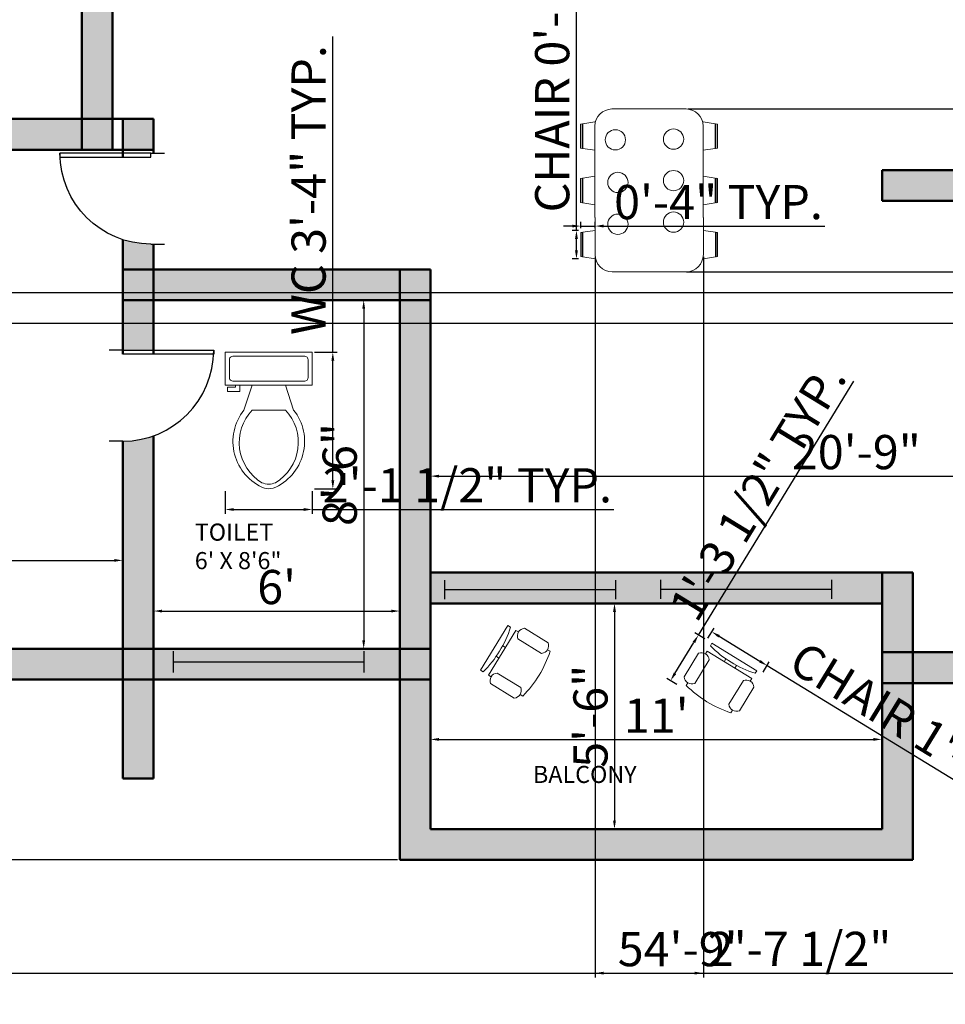
# Model space of a CAD drawing. Units: millimetres. Extents: x 2208 to 3043, y 878 to 1386.
# Tile 2 of 4: x 2479 to 2749, y 878 to 1166. Entities that reach past the tile are written whole.
import ezdxf

# ---------------------------------------------------------------- set-up
doc = ezdxf.new("R2010")
doc.units = ezdxf.units.MM
for name, color, linetype, lineweight in [('A-ANNO-DIMS', 50, 'Continuous', 13), ('A-AREA-IDEN', 90, 'Continuous', 25), ('A-FLOR-FIXT', 140, 'Continuous', 18), ('A-WALL-PATT', 6, 'Continuous', 13), ('doors', 30, 'Continuous', 25), ('furniture', 140, 'Continuous', 18), ('walls', 200, 'Continuous', 50), ('windows', 10, 'Continuous', 25)]:
    doc.layers.add(name, color=color, linetype=linetype, lineweight=lineweight)
doc.styles.get("Standard").update_dxf_attribs({"font": 'arial.ttf'})
doc.dimstyles.new('ISO-25', dxfattribs={"dimtxt": 10, "dimasz": 2.5, "dimexe": 1.25, "dimexo": 0.625, "dimtad": 1, "dimdec": 0, "dimlunit": 3, "dimtxsty": 'Standard', "dimcen": 2.5, "dimadec": 0, "dimazin": 0, "dimtfac": 1, "dimtdec": 0, "dimtmove": 0, "dimatfit": 3, "dimfxl": 1, "dimarcsym": 0})

# ---------------------------------------------------------------- blocks, each defined once
blk = doc.blocks.new('*U2')
for p, q in [((0, 0), (0, -6)), ((40, 0), (40, -6))]:
    blk.add_line(p, q)
blk.add_lwpolyline([(0, 0), (0, 40), (1.75, 40), (1.75, 0)], close=True)
blk.add_arc((0, 0), 40, 0, 90)
blk = doc.blocks.new('*U4')
for p, q in [((0, 4), (0, 0)), ((36, 4), (36, 0)), ((0, 2), (36, 2))]:
    blk.add_line(p, q)
blk = doc.blocks.new('*U5')
for p, q in [((0, 4), (0, 0)), ((36, 4), (36, 0)), ((0, 2), (36, 2))]:
    blk.add_line(p, q)
blk = doc.blocks.new('Chair - Desk')
for p, q in [((-8.5, 0), (-8.5, -1)), ((-8.5, 0), (8.5, 0)), ((8.5, 0), (8.5, -1)), ((-8.5, -3), (-8.5, -4)), ((-8.5, -3), (8.5, -3)), ((-2, -3), (-2, -1.9355)), ((2, -1.9576), (2, -3)), ((8.5, -3), (8.5, -4)), ((-10.5, -5), (-10.5, -14)), ((-6.5, -14), (-6.5, -5)), ((6.5, -5), (6.5, -14)), ((10.5, -14), (10.5, -5)), ((-8.5, -15), (-8.5, -16)), ((8.5, -15), (8.5, -16))]:
    blk.add_line(p, q)
for centre, radius, start, end in [((0, 34.625), 36.625, 256.5803, 283.4197), ((-8.5, -6.5), 2.5, 36.8699, 143.1301), ((8.5, -6.5), 2.5, 36.8699, 143.1301), ((-8.5, -12.5), 2.5, 216.8699, 323.1301), ((8.5, -12.5), 2.5, 216.8699, 323.1301), ((0, 19.625), 36.625, 256.5803, 283.4197)]:
    blk.add_arc(centre, radius, start, end)
blk = doc.blocks.new('Toilet - top')
for p, q in [((9.5, -6), (9.5, -2)), ((-10, -8.5), (-8, -8.5)), ((-10, -9.5), (-10, -8.5)), ((-7, -9.5), (-10, -9.5)), ((-8, -8.5), (-8, -8)), ((-7, -8), (-7, -9.5)), ((-4, -8), (-6, -14)), ((4, -8), (6, -14)), ((4, -14), (-4, -14))]:
    blk.add_line(p, q)
blk.add_lwpolyline([(10.5, -8), (10.5, 0), (-10.5, 0), (-10.5, -8)], close=True)
for points in [[(-9.5, -2), (-9.5, -6)], [(8.5, -1), (-8.5, -1)], [(-8.5, -7), (8.5, -7)]]:
    blk.add_lwpolyline(points)
for centre, radius, start, end in [((-8.62, -1.88), 0.884, 81.8699, 188.1301), ((8.62, -1.88), 0.884, 351.8699, 98.1301), ((-8.62, -6.12), 0.884, 171.8699, 278.1301), ((8.62, -6.12), 0.884, 261.8699, 8.1301), ((3.52, -21.58), 12.17, 141.4691, 247.9714), ((4.2, -21.82), 11.33, 136.3677, 238.9468), ((-3.52, -21.58), 12.17, 292.0284, 38.5307), ((-4.2, -21.82), 11.33, 301.053, 43.6321), ((0, -27.88), 4, 245.7318, 294.2682), ((0, -29), 4, 254.8605, 285.1395)]:
    blk.add_arc(centre, radius, start, end)
blk = doc.blocks.new('*D22')
at = {"layer": 'A-ANNO-DIMS', "color": 0, "lineweight": -2, "transparency": 16777216}
for p, q in [((2352.98, 996.86), (2352.98, 1009.56)), ((2355.48, 1008.31), (2506.48, 1008.31)), ((2508.98, 996.86), (2508.98, 1009.56))]:
    blk.add_line(p, q, dxfattribs=at)
at = {"layer": 'A-ANNO-DIMS', "color": 0, "transparency": 16777216}
for points in [[(2355.48, 1008.73), (2355.48, 1007.9), (2352.98, 1008.31)], [(2506.48, 1008.73), (2506.48, 1007.9), (2508.98, 1008.31)]]:
    blk.add_solid(points, dxfattribs=at)
at = {"layer": 'Defpoints', "color": 0, "transparency": 16777216}
for p in [(2508.98, 1008.31), (2352.98, 996.23), (2508.98, 996.23)]:
    blk.add_point(p, dxfattribs=at)
at = {"layer": 'A-ANNO-DIMS', "color": 0, "transparency": 16777216, "insert": (2430.98, 1014.05), "char_height": 10, "attachment_point": 5}
blk.add_mtext("13'", dxfattribs=at)
blk = doc.blocks.new('*D23')
at = {"layer": 'A-ANNO-DIMS', "color": 0, "lineweight": -2, "transparency": 16777216}
for p, q in [((2517.98, 1002.61), (2517.98, 992.24)), ((2589.98, 1002.61), (2589.98, 992.24)), ((2520.48, 993.49), (2587.48, 993.49))]:
    blk.add_line(p, q, dxfattribs=at)
at = {"layer": 'A-ANNO-DIMS', "color": 0, "transparency": 16777216}
for points in [[(2520.48, 993.9), (2520.48, 993.07), (2517.98, 993.49)], [(2587.48, 993.9), (2587.48, 993.07), (2589.98, 993.49)]]:
    blk.add_solid(points, dxfattribs=at)
at = {"layer": 'Defpoints', "color": 0, "transparency": 16777216}
for p in [(2517.98, 1003.23), (2589.98, 1003.23), (2589.98, 993.49)]:
    blk.add_point(p, dxfattribs=at)
at = {"layer": 'A-ANNO-DIMS', "color": 0, "transparency": 16777216, "insert": (2553.98, 999.22), "char_height": 10, "attachment_point": 5}
blk.add_mtext("6'", dxfattribs=at)
blk = doc.blocks.new('*D24')
at = {"layer": 'A-ANNO-DIMS', "color": 0, "lineweight": -2, "transparency": 16777216}
for p, q in [((2582.68, 1084.44), (2578.18, 1084.44)), ((2579.43, 1081.94), (2579.43, 984.94)), ((2582.68, 982.44), (2578.18, 982.44))]:
    blk.add_line(p, q, dxfattribs=at)
at = {"layer": 'A-ANNO-DIMS', "color": 0, "transparency": 16777216}
for points in [[(2579.01, 1081.94), (2579.85, 1081.94), (2579.43, 1084.44)], [(2579.01, 984.94), (2579.85, 984.94), (2579.43, 982.44)]]:
    blk.add_solid(points, dxfattribs=at)
at = {"layer": 'Defpoints', "color": 0, "transparency": 16777216}
for p in [(2583.3, 1084.44), (2579.43, 982.44), (2583.3, 982.44)]:
    blk.add_point(p, dxfattribs=at)
at = {"layer": 'A-ANNO-DIMS', "color": 0, "transparency": 16777216, "insert": (2573.7, 1033.44), "char_height": 10, "attachment_point": 5, "rotation": 90}
blk.add_mtext('8\'-6"', dxfattribs=at)
blk = doc.blocks.new('*D25')
at = {"layer": 'A-ANNO-DIMS', "color": 0, "lineweight": -2, "transparency": 16777216}
for p, q in [((2598.98, 952.2), (2598.98, 957.19)), ((2730.98, 952.2), (2730.98, 957.19)), ((2601.48, 955.94), (2728.48, 955.94))]:
    blk.add_line(p, q, dxfattribs=at)
at = {"layer": 'A-ANNO-DIMS', "color": 0, "transparency": 16777216}
for points in [[(2601.48, 956.36), (2601.48, 955.53), (2598.98, 955.94)], [(2728.48, 956.36), (2728.48, 955.53), (2730.98, 955.94)]]:
    blk.add_solid(points, dxfattribs=at)
at = {"layer": 'Defpoints', "color": 0, "transparency": 16777216}
for p in [(2730.98, 955.94), (2598.98, 951.58), (2730.98, 951.58)]:
    blk.add_point(p, dxfattribs=at)
at = {"layer": 'A-ANNO-DIMS', "color": 0, "transparency": 16777216, "insert": (2664.98, 961.59), "char_height": 10, "attachment_point": 5}
blk.add_mtext("11'", dxfattribs=at)
blk = doc.blocks.new('*D26')
at = {"layer": 'A-ANNO-DIMS', "color": 0, "lineweight": -2, "transparency": 16777216}
for p, q in [((2657.86, 995.72), (2651.51, 995.72)), ((2652.76, 993.22), (2652.76, 932.22)), ((2657.86, 929.72), (2651.51, 929.72))]:
    blk.add_line(p, q, dxfattribs=at)
at = {"layer": 'A-ANNO-DIMS', "color": 0, "transparency": 16777216}
for points in [[(2652.34, 993.22), (2653.18, 993.22), (2652.76, 995.72)], [(2652.34, 932.22), (2653.18, 932.22), (2652.76, 929.72)]]:
    blk.add_solid(points, dxfattribs=at)
at = {"layer": 'Defpoints', "color": 0, "transparency": 16777216}
for p in [(2658.49, 995.72), (2652.76, 929.72), (2658.49, 929.72)]:
    blk.add_point(p, dxfattribs=at)
at = {"layer": 'A-ANNO-DIMS', "color": 0, "transparency": 16777216, "insert": (2647.03, 962.72), "char_height": 10, "attachment_point": 5, "rotation": 90}
blk.add_mtext('5\'-6"', dxfattribs=at)
blk = doc.blocks.new('*D27')
at = {"layer": 'A-ANNO-DIMS', "color": 0, "lineweight": -2, "transparency": 16777216}
for p, q in [((2598.98, 1051.4), (2598.98, 1031.71)), ((2847.98, 1051.4), (2847.98, 1031.71)), ((2601.48, 1032.96), (2845.48, 1032.96))]:
    blk.add_line(p, q, dxfattribs=at)
at = {"layer": 'A-ANNO-DIMS', "color": 0, "transparency": 16777216}
for points in [[(2601.48, 1033.38), (2601.48, 1032.54), (2598.98, 1032.96)], [(2845.48, 1033.38), (2845.48, 1032.54), (2847.98, 1032.96)]]:
    blk.add_solid(points, dxfattribs=at)
at = {"layer": 'Defpoints', "color": 0, "transparency": 16777216}
for p in [(2598.98, 1052.02), (2847.98, 1052.02), (2847.98, 1032.96)]:
    blk.add_point(p, dxfattribs=at)
at = {"layer": 'A-ANNO-DIMS', "color": 0, "transparency": 16777216, "insert": (2723.48, 1038.69), "char_height": 10, "attachment_point": 5}
blk.add_mtext('20\'-9"', dxfattribs=at)
blk = doc.blocks.new('CHAIR-DINING')
for p, q in [((0, 7.69), (0.44, 7.76)), ((0, 7.69), (0, 0.65)), ((0.44, 0.58), (0.44, 7.76)), ((0.66, 7.79), (4.18, 8.34)), ((0.66, 7.79), (0.66, 0.55)), ((0.44, 0.58), (0, 0.65)), ((4.18, 0), (0.66, 0.55))]:
    blk.add_line(p, q)
blk = doc.blocks.new('*D34')
at = {"layer": 'A-ANNO-DIMS', "color": 0, "lineweight": -2, "transparency": 16777216}
for p, q in [((2641.64, 1104.85), (2641.64, 1240.09)), ((2642.27, 1104.85), (2640.39, 1104.85)), ((2641.64, 1099.01), (2641.64, 1102.35)), ((2642.27, 1096.51), (2640.39, 1096.51))]:
    blk.add_line(p, q, dxfattribs=at)
at = {"layer": 'A-ANNO-DIMS', "color": 0, "transparency": 16777216}
for points in [[(2641.22, 1102.35), (2642.06, 1102.35), (2641.64, 1104.85)], [(2641.22, 1099.01), (2642.06, 1099.01), (2641.64, 1096.51)]]:
    blk.add_solid(points, dxfattribs=at)
at = {"layer": 'Defpoints', "color": 0, "transparency": 16777216}
for p in [(2641.64, 1104.85), (2642.89, 1104.85), (2642.89, 1096.51)]:
    blk.add_point(p, dxfattribs=at)
at = {"layer": 'A-ANNO-DIMS', "color": 0, "transparency": 16777216, "insert": (2635.84, 1173.72), "char_height": 10, "attachment_point": 5, "rotation": 90}
blk.add_mtext('CHAIR 0\'-8 1/2" TYP.', dxfattribs=at)
blk = doc.blocks.new('*D35')
at = {"layer": 'A-ANNO-DIMS', "color": 0, "lineweight": -2, "transparency": 16777216}
for p, q in [((2640.39, 1106.1), (2637.89, 1106.1)), ((2642.89, 1105.48), (2642.89, 1107.35)), ((2642.89, 1106.1), (2647.07, 1106.1)), ((2647.07, 1105.48), (2647.07, 1107.35)), ((2649.57, 1106.1), (2714.28, 1106.1))]:
    blk.add_line(p, q, dxfattribs=at)
at = {"layer": 'A-ANNO-DIMS', "color": 0, "transparency": 16777216}
for points in [[(2640.39, 1106.52), (2640.39, 1105.69), (2642.89, 1106.1)], [(2649.57, 1106.52), (2649.57, 1105.69), (2647.07, 1106.1)]]:
    blk.add_solid(points, dxfattribs=at)
at = {"layer": 'Defpoints', "color": 0, "transparency": 16777216}
for p in [(2647.07, 1106.1), (2642.89, 1104.85), (2647.07, 1104.85)]:
    blk.add_point(p, dxfattribs=at)
at = {"layer": 'A-ANNO-DIMS', "color": 0, "transparency": 16777216, "insert": (2683.17, 1111.83), "char_height": 10, "attachment_point": 5}
blk.add_mtext('0\'-4" TYP.', dxfattribs=at)
blk = doc.blocks.new('*D38')
at = {"layer": 'A-ANNO-DIMS', "color": 0, "lineweight": -2, "transparency": 16777216}
for p, q in [((2680.05, 985.52), (2681.86, 988.48)), ((2683.34, 986.11), (2695.25, 978.83)), ((2696.22, 975.63), (2698.03, 978.59)), ((2697.38, 977.52), (2792.87, 919.11))]:
    blk.add_line(p, q, dxfattribs=at)
at = {"layer": 'A-ANNO-DIMS', "color": 0, "transparency": 16777216}
for points in [[(2683.56, 986.47), (2683.13, 985.76), (2681.21, 987.42)], [(2695.47, 979.18), (2695.03, 978.47), (2697.38, 977.52)]]:
    blk.add_solid(points, dxfattribs=at)
at = {"layer": 'Defpoints', "color": 0, "transparency": 16777216}
for p in [(2679.73, 984.99), (2697.38, 977.52), (2695.9, 975.1)]:
    blk.add_point(p, dxfattribs=at)
at = {"layer": 'A-ANNO-DIMS', "color": 0, "transparency": 16777216, "insert": (2749.21, 952.61), "char_height": 10, "attachment_point": 5, "rotation": 328.5439}
blk.add_mtext('CHAIR 1\'-7" TYP.', dxfattribs=at)
blk = doc.blocks.new('*D39')
at = {"layer": 'A-ANNO-DIMS', "color": 0, "lineweight": -2, "transparency": 16777216}
for p, q in [((2677.3, 986.48), (2722.74, 1060.75)), ((2679.19, 985.32), (2676.24, 987.13)), ((2670.44, 975.26), (2676, 984.34)), ((2671.03, 971.97), (2668.07, 973.78))]:
    blk.add_line(p, q, dxfattribs=at)
at = {"layer": 'A-ANNO-DIMS', "color": 0, "transparency": 16777216}
for points in [[(2675.64, 984.56), (2676.35, 984.13), (2677.3, 986.48)], [(2670.09, 975.48), (2670.8, 975.04), (2669.14, 973.13)]]:
    blk.add_solid(points, dxfattribs=at)
at = {"layer": 'Defpoints', "color": 0, "transparency": 16777216}
for p in [(2677.3, 986.48), (2679.73, 984.99), (2671.56, 971.64)]:
    blk.add_point(p, dxfattribs=at)
at = {"layer": 'A-ANNO-DIMS', "color": 0, "transparency": 16777216, "insert": (2695.72, 1027.7), "char_height": 10, "attachment_point": 5, "rotation": 58.5439}
blk.add_mtext('1\'-3 1/2" TYP.', dxfattribs=at)
blk = doc.blocks.new('*D40')
at = {"layer": 'A-ANNO-DIMS', "color": 0, "lineweight": -2, "transparency": 16777216}
for p, q in [((2570.4, 1069.24), (2570.4, 1161.51)), ((2565.02, 1069.24), (2571.65, 1069.24)), ((2570.4, 1031.7), (2570.4, 1066.74)), ((2565.02, 1029.2), (2571.65, 1029.2))]:
    blk.add_line(p, q, dxfattribs=at)
at = {"layer": 'A-ANNO-DIMS', "color": 0, "transparency": 16777216}
for points in [[(2569.99, 1066.74), (2570.82, 1066.74), (2570.4, 1069.24)], [(2569.99, 1031.7), (2570.82, 1031.7), (2570.4, 1029.2)]]:
    blk.add_solid(points, dxfattribs=at)
at = {"layer": 'Defpoints', "color": 0, "transparency": 16777216}
for p in [(2564.4, 1069.24), (2570.4, 1069.24), (2564.4, 1029.2)]:
    blk.add_point(p, dxfattribs=at)
at = {"layer": 'A-ANNO-DIMS', "color": 0, "transparency": 16777216, "insert": (2564.61, 1116.63), "char_height": 10, "attachment_point": 5, "rotation": 90}
blk.add_mtext('WC 3\'-4" TYP.', dxfattribs=at)
blk = doc.blocks.new('*D41')
at = {"layer": 'A-ANNO-DIMS', "color": 0, "lineweight": -2, "transparency": 16777216}
for p, q in [((2538.95, 1028.57), (2538.95, 1021.94)), ((2564.4, 1028.57), (2564.4, 1021.94)), ((2541.45, 1023.19), (2561.9, 1023.19)), ((2564.4, 1023.19), (2652.58, 1023.19))]:
    blk.add_line(p, q, dxfattribs=at)
at = {"layer": 'A-ANNO-DIMS', "color": 0, "transparency": 16777216}
for points in [[(2541.45, 1023.61), (2541.45, 1022.78), (2538.95, 1023.19)], [(2561.9, 1023.61), (2561.9, 1022.78), (2564.4, 1023.19)]]:
    blk.add_solid(points, dxfattribs=at)
at = {"layer": 'Defpoints', "color": 0, "transparency": 16777216}
for p in [(2538.95, 1029.2), (2564.4, 1029.2), (2564.4, 1023.19)]:
    blk.add_point(p, dxfattribs=at)
at = {"layer": 'A-ANNO-DIMS', "color": 0, "transparency": 16777216, "insert": (2609.74, 1028.99), "char_height": 10, "attachment_point": 5}
blk.add_mtext('2\'-1 1/2" TYP.', dxfattribs=at)
blk = doc.blocks.new('*D46')
at = {"layer": 'A-ANNO-DIMS', "color": 0, "lineweight": -2, "transparency": 16777216}
for p, q in [((3001.16, 1077), (3001.16, 886.32)), ((2343.98, 972.81), (2343.98, 886.32)), ((2346.48, 887.57), (2998.66, 887.57))]:
    blk.add_line(p, q, dxfattribs=at)
at = {"layer": 'A-ANNO-DIMS', "color": 0, "transparency": 16777216}
for points in [[(2346.48, 887.99), (2346.48, 887.16), (2343.98, 887.57)], [(2998.66, 887.99), (2998.66, 887.16), (3001.16, 887.57)]]:
    blk.add_solid(points, dxfattribs=at)
at = {"layer": 'Defpoints', "color": 0, "transparency": 16777216}
for p in [(3001.16, 1077.62), (2343.98, 973.44), (3001.16, 887.57)]:
    blk.add_point(p, dxfattribs=at)
at = {"layer": 'A-ANNO-DIMS', "color": 0, "transparency": 16777216, "insert": (2672.57, 893.3), "char_height": 10, "attachment_point": 5}
blk.add_mtext('54\'-9"', dxfattribs=at)
blk = doc.blocks.new('*D47')
at = {"layer": 'A-ANNO-DIMS', "color": 0, "lineweight": -2, "transparency": 16777216}
for p, q in [((2343.36, 1332.44), (2309.12, 1332.44)), ((2310.37, 1329.94), (2310.37, 923.22)), ((2589.36, 920.72), (2309.12, 920.72))]:
    blk.add_line(p, q, dxfattribs=at)
at = {"layer": 'A-ANNO-DIMS', "color": 0, "transparency": 16777216}
for points in [[(2309.95, 1329.94), (2310.79, 1329.94), (2310.37, 1332.44)], [(2309.95, 923.22), (2310.79, 923.22), (2310.37, 920.72)]]:
    blk.add_solid(points, dxfattribs=at)
at = {"layer": 'Defpoints', "color": 0, "transparency": 16777216}
for p in [(2343.98, 1332.44), (2310.37, 920.72), (2589.98, 920.72)]:
    blk.add_point(p, dxfattribs=at)
at = {"layer": 'A-ANNO-DIMS', "color": 0, "transparency": 16777216, "insert": (2304.57, 1126.58), "char_height": 10, "attachment_point": 5, "rotation": 90}
blk.add_mtext('34\'-3 1/2"', dxfattribs=at)
blk = doc.blocks.new('*D62')
at = {"layer": 'A-ANNO-DIMS', "color": 0, "lineweight": -2, "transparency": 16777216}
for p, q in [((2310.37, 1086.62), (2310.37, 1116.95)), ((3000.54, 1086.62), (2309.12, 1086.62)), ((2310.37, 1080.12), (2310.37, 1084.12)), ((3000.54, 1077.62), (2309.12, 1077.62))]:
    blk.add_line(p, q, dxfattribs=at)
at = {"layer": 'A-ANNO-DIMS', "color": 0, "transparency": 16777216}
for points in [[(2309.95, 1084.12), (2310.79, 1084.12), (2310.37, 1086.62)], [(2309.95, 1080.12), (2310.79, 1080.12), (2310.37, 1077.62)]]:
    blk.add_solid(points, dxfattribs=at)
at = {"layer": 'Defpoints', "color": 0, "transparency": 16777216}
for p in [(2310.37, 1086.62), (3001.16, 1086.62), (3001.16, 1077.62)]:
    blk.add_point(p, dxfattribs=at)
at = {"layer": 'A-ANNO-DIMS', "color": 0, "transparency": 16777216, "insert": (2304.64, 1103.04), "char_height": 10, "attachment_point": 5, "rotation": 90}
blk.add_mtext('0\'-9"', dxfattribs=at)
blk = doc.blocks.new('*D65')
at = {"layer": 'A-ANNO-DIMS', "color": 0, "lineweight": -2, "transparency": 16777216}
for p, q in [((2647.07, 1097.14), (2647.07, 886.32)), ((2678.74, 1097.14), (2678.74, 886.32)), ((2649.57, 887.57), (2676.24, 887.57)), ((2678.74, 887.57), (2732.54, 887.57))]:
    blk.add_line(p, q, dxfattribs=at)
at = {"layer": 'A-ANNO-DIMS', "color": 0, "transparency": 16777216}
for points in [[(2649.57, 887.99), (2649.57, 887.16), (2647.07, 887.57)], [(2676.24, 887.99), (2676.24, 887.16), (2678.74, 887.57)]]:
    blk.add_solid(points, dxfattribs=at)
at = {"layer": 'Defpoints', "color": 0, "transparency": 16777216}
for p in [(2647.07, 1097.76), (2678.74, 1097.76), (2678.74, 887.57)]:
    blk.add_point(p, dxfattribs=at)
at = {"layer": 'A-ANNO-DIMS', "color": 0, "transparency": 16777216, "insert": (2706.89, 893.37), "char_height": 10, "attachment_point": 5}
blk.add_mtext('2\'-7 1/2"', dxfattribs=at)
blk = doc.blocks.new('*D66')
at = {"layer": 'A-ANNO-DIMS', "color": 0, "lineweight": -2, "transparency": 16777216}
for p, q in [((3034.31, 1140.35), (3034.31, 1201.74)), ((2674.33, 1140.35), (3035.56, 1140.35)), ((3034.31, 1095.26), (3034.31, 1137.85)), ((2673.86, 1092.76), (3035.56, 1092.76))]:
    blk.add_line(p, q, dxfattribs=at)
at = {"layer": 'A-ANNO-DIMS', "color": 0, "transparency": 16777216}
for points in [[(3033.9, 1137.85), (3034.73, 1137.85), (3034.31, 1140.35)], [(3033.9, 1095.26), (3034.73, 1095.26), (3034.31, 1092.76)]]:
    blk.add_solid(points, dxfattribs=at)
at = {"layer": 'Defpoints', "color": 0, "transparency": 16777216}
for p in [(2673.7, 1140.35), (3034.31, 1140.35), (2673.23, 1092.76)]:
    blk.add_point(p, dxfattribs=at)
at = {"layer": 'A-ANNO-DIMS', "color": 0, "transparency": 16777216, "insert": (3028.52, 1172.3), "char_height": 10, "attachment_point": 5, "rotation": 90}
blk.add_mtext('3\'-11 1/2"', dxfattribs=at)

msp = doc.modelspace()

# ---------------------------------------------------------------- hatches: boundary and pattern name
at = {"layer": 'A-WALL-PATT'}
h = msp.add_hatch(color=256, dxfattribs=at)
h.dxf.hatch_style = 1
h.paths.add_polyline_path([(2352.98, 1273, -0.051847), (2347.51, 1272.43), (2343.98, 1272.43), (2343.98, 1137.44), (2352.98, 1137.44)])
h.paths.add_polyline_path([(2352.98, 1323.44), (2343.98, 1323.44), (2343.98, 1299.03), (2347.51, 1299.03), (2352.98, 1299.03)])
h.paths.add_polyline_path([(2352.98, 1332.44), (2343.98, 1332.44), (2343.98, 1323.44), (2352.98, 1323.44)])
h.paths.add_polyline_path([(2496.98, 1332.44), (2352.98, 1332.44), (2352.98, 1323.44), (2496.98, 1323.44)])
h.paths.add_polyline_path([(2505.98, 1323.44), (2496.98, 1323.44), (2496.98, 1191.44), (2505.98, 1191.44)])
h.paths.add_polyline_path([(2505.98, 1332.44), (2496.98, 1332.44), (2496.98, 1323.44), (2505.98, 1323.44)])
h.paths.add_polyline_path([(2505.98, 1182.44), (2496.98, 1182.44), (2496.98, 1137.44), (2505.98, 1137.44)])
h.paths.add_polyline_path([(2505.98, 1191.44), (2496.98, 1191.44), (2496.98, 1182.44), (2505.98, 1182.44)])
h.paths.add_polyline_path([(2621.06, 1191.44), (2505.98, 1191.44), (2505.98, 1182.44), (2619.92, 1182.44), (2619.92, 1183.73, -0.073589)])
h.paths.add_polyline_path([(2496.98, 1137.44), (2352.98, 1137.44), (2352.98, 1128.44), (2496.98, 1128.44)])
h.paths.add_polyline_path([(2352.98, 1137.44), (2343.98, 1137.44), (2343.98, 1128.44), (2352.98, 1128.44)])
h.paths.add_polyline_path([(2352.98, 1128.44), (2343.98, 1128.44), (2343.98, 982.44), (2352.98, 982.44)])
h.paths.add_polyline_path([(2517.98, 1137.44), (2508.98, 1137.44), (2508.98, 1128.44), (2517.98, 1128.44)])
h.paths.add_polyline_path([(2505.98, 1137.44), (2496.98, 1137.44), (2496.98, 1128.44), (2505.98, 1128.44)])
h.paths.add_polyline_path([(2658.98, 1224.44), (2649.98, 1224.44), (2649.98, 1191.44), (2658.98, 1191.44)])
h.paths.add_polyline_path([(2658.98, 1323.44), (2649.98, 1323.44), (2649.98, 1233.44), (2658.98, 1233.44)])
h.paths.add_polyline_path([(2658.98, 1233.44), (2649.98, 1233.44), (2649.98, 1224.44), (2658.98, 1224.44)])
h.paths.add_polyline_path([(2730.98, 1233.44), (2658.98, 1233.44), (2658.98, 1224.44), (2730.98, 1224.44)])
h.paths.add_polyline_path([(2739.98, 1323.44), (2730.98, 1323.44), (2730.98, 1233.44), (2739.98, 1233.44)])
h.paths.add_polyline_path([(2739.98, 1224.44), (2730.98, 1224.44), (2730.98, 1191.44), (2739.98, 1191.44)])
h.paths.add_polyline_path([(2739.98, 1191.44), (2730.98, 1191.44), (2730.98, 1182.44), (2739.98, 1182.44)])
h.paths.add_polyline_path([(2739.98, 1182.44), (2730.98, 1182.44), (2730.98, 1171.44), (2739.98, 1171.44)])
h.paths.add_polyline_path([(2739.98, 972.44), (2730.98, 972.44), (2730.98, 929.72), (2602.15, 929.72), (2598.98, 929.72), (2598.98, 973.44), (2589.98, 973.44), (2589.98, 929.72), (2589.98, 920.72), (2730.98, 920.72), (2739.98, 920.72)])
h.paths.add_polyline_path([(2598.98, 1084.44), (2589.98, 1084.44), (2589.98, 982.44), (2598.98, 982.44)])
h.paths.add_polyline_path([(2598.98, 982.44), (2589.98, 982.44), (2589.98, 973.44), (2598.98, 973.44)])
h.paths.add_polyline_path([(2517.98, 973.44), (2508.98, 973.44), (2508.98, 944.53), (2517.98, 944.53)])
h.paths.add_polyline_path([(2517.98, 1044.76, -0.086498), (2508.98, 1043.19), (2508.98, 982.44), (2517.98, 982.44)])
h.paths.add_polyline_path([(2517.98, 982.44), (2508.98, 982.44), (2508.98, 973.44), (2517.98, 973.44)])
h.paths.add_polyline_path([(2352.98, 982.44), (2343.98, 982.44), (2343.98, 973.44), (2352.98, 973.44)])
h.paths.add_polyline_path([(2589.98, 1093.44), (2517.98, 1093.44), (2517.98, 1084.44), (2589.98, 1084.44)])
h.paths.add_polyline_path([(2517.98, 1093.44), (2508.98, 1093.44), (2508.98, 1084.44), (2517.98, 1084.44)])
h.paths.add_polyline_path([(2517.98, 1084.44), (2508.98, 1084.44), (2508.98, 1069.79), (2517.98, 1069.79)])
h.paths.add_polyline_path([(2517.98, 1100.83), (2517.21, 1100.83, -0.078775), (2508.98, 1102.14), (2508.98, 1093.44), (2517.98, 1093.44)])
h.paths.add_polyline_path([(2598.98, 1093.44), (2589.98, 1093.44), (2589.98, 1084.44), (2598.98, 1084.44)])
h.paths.add_polyline_path([(2802.98, 1122.44), (2730.98, 1122.44), (2730.98, 1113.44), (2802.98, 1113.44)])
h.paths.add_polyline_path([(2922.98, 1113.44), (2913.98, 1113.44), (2913.98, 981.44), (2922.98, 981.44)])
h.paths.add_polyline_path([(2856.98, 1069.77, -0.087206), (2847.98, 1067.81), (2847.98, 981.44), (2856.98, 981.44)])
h.paths.add_polyline_path([(2913.98, 981.44), (2856.98, 981.44), (2856.98, 972.44), (2913.98, 972.44)])
h.paths.add_polyline_path([(2856.98, 981.44), (2847.98, 981.44), (2847.98, 972.44), (2856.98, 972.44)])
h.paths.add_polyline_path([(2739.98, 995.72), (2739.98, 1004.72), (2730.98, 1004.72), (2730.98, 981.44), (2739.98, 981.44)])
h.paths.add_polyline_path([(2739.98, 981.44), (2730.98, 981.44), (2730.98, 972.44), (2739.98, 972.44)])
h.paths.add_polyline_path([(2922.98, 981.44), (2913.98, 981.44), (2913.98, 972.44), (2922.98, 972.44)])
h.paths.add_polyline_path([(3001.16, 1086.62), (2922.98, 1086.62), (2922.98, 1077.62), (3001.16, 1077.62)])
h.paths.add_polyline_path([(3001.16, 1191.44), (2922.98, 1191.44), (2922.98, 1182.44), (3001.16, 1182.44)])
h.paths.add_polyline_path([(2913.98, 1191.44), (2843.61, 1191.44), (2843.49, 1188.69, -0.05974), (2842.46, 1182.44), (2913.98, 1182.44)])
h.paths.add_polyline_path([(2922.98, 1191.44), (2913.98, 1191.44), (2913.98, 1182.44), (2922.98, 1182.44)])
h.paths.add_polyline_path([(2802.98, 1191.44), (2769.17, 1191.44, -0.079558), (2770.5, 1183.13), (2770.5, 1182.44), (2802.98, 1182.44)])
h.paths.add_polyline_path([(2811.98, 1191.44), (2802.98, 1191.44), (2802.98, 1182.44), (2811.98, 1182.44)])
h.paths.add_polyline_path([(2811.98, 1182.44), (2802.98, 1182.44), (2802.98, 1122.44), (2811.98, 1122.44)])
h.paths.add_polyline_path([(2811.98, 1122.44), (2802.98, 1122.44), (2802.98, 1113.44), (2811.98, 1113.44)])
h.paths.add_polyline_path([(2847.98, 1122.44), (2811.98, 1122.44), (2811.98, 1113.44), (2847.98, 1113.44)])
h.paths.add_polyline_path([(2856.98, 1122.44), (2847.98, 1122.44), (2847.98, 1113.44), (2856.98, 1113.44)])
h.paths.add_polyline_path([(2913.98, 1122.44), (2856.98, 1122.44), (2856.98, 1113.44), (2913.98, 1113.44)])
h.paths.add_polyline_path([(2922.98, 1122.44), (2913.98, 1122.44), (2913.98, 1113.44), (2922.98, 1113.44)])
h.paths.add_polyline_path([(2856.98, 1113.44), (2847.98, 1113.44), (2847.98, 1094.39), (2856.98, 1094.39)])
h.paths.add_polyline_path([(2922.98, 1323.44), (2913.98, 1323.44), (2913.98, 1191.44), (2922.98, 1191.44)])
h.paths.add_polyline_path([(2922.98, 1332.44), (2913.98, 1332.44), (2913.98, 1323.44), (2922.98, 1323.44)])
h.paths.add_polyline_path([(2913.98, 1332.44), (2739.98, 1332.44), (2739.98, 1323.44), (2913.98, 1323.44)])
h.paths.add_polyline_path([(2730.98, 1332.44), (2658.98, 1332.44), (2658.98, 1323.44), (2730.98, 1323.44)])
h.paths.add_polyline_path([(2649.98, 1332.44), (2505.98, 1332.44), (2505.98, 1323.44), (2649.98, 1323.44)])
h.paths.add_polyline_path([(2658.98, 1332.44), (2649.98, 1332.44), (2649.98, 1323.44), (2658.98, 1323.44)])
h.paths.add_polyline_path([(2739.98, 1332.44), (2730.98, 1332.44), (2730.98, 1323.44), (2739.98, 1323.44)])
h.paths.add_polyline_path([(2739.98, 1233.44), (2730.98, 1233.44), (2730.98, 1224.44), (2739.98, 1224.44)])
h.paths.add_polyline_path([(2658.98, 1191.44), (2649.98, 1191.44), (2649.98, 1182.44), (2658.98, 1182.44)])
h.paths.add_polyline_path([(2658.98, 1182.44), (2649.98, 1182.44), (2649.98, 1171.44), (2658.98, 1171.44)])
h.paths.add_polyline_path([(2508.98, 982.44), (2352.98, 982.44), (2352.98, 973.44), (2508.98, 973.44)])
h.paths.add_polyline_path([(2589.98, 982.44), (2517.98, 982.44), (2517.98, 973.44), (2589.98, 973.44)])
h.paths.add_polyline_path([(2730.98, 1004.72), (2598.98, 1004.72), (2598.98, 995.72), (2730.98, 995.72)])
h.paths.add_polyline_path([(2847.98, 981.44), (2739.98, 981.44), (2739.98, 972.44), (2847.98, 972.44)])

# ---------------------------------------------------------------- linework, layer by layer
at = {"layer": 'furniture'}
for p, q in [((2673.7, 1140.35), (2652.03, 1140.35)), ((2647.03, 1135.35), (2647.03, 1124.51)), ((2678.7, 1124.51), (2678.7, 1135.35)), ((2647.05, 1124.44), (2647.05, 1108.61)), ((2678.71, 1108.61), (2678.71, 1124.44)), ((2647.07, 1108.6), (2647.07, 1097.76)), ((2678.74, 1097.76), (2678.74, 1108.6)), ((2652.07, 1092.76), (2673.74, 1092.76)), ((2652.57, 1092.76), (2652.57, 1092.76)), ((2660.92, 1092.76), (2660.92, 1092.76)), ((2664.89, 1092.76), (2664.89, 1092.76)), ((2673.23, 1092.76), (2673.23, 1092.76))]:
    msp.add_line(p, q, dxfattribs=at)
for centre in [(2653.02, 1131.33), (2670.03, 1131.54), (2653.76, 1118.87), (2670.03, 1119.4), (2653.76, 1106.63), (2670.03, 1107.26)]:
    msp.add_circle(centre, 2.97, dxfattribs=at)
for centre, start, end in [((2652.03, 1135.35), 90, 180), ((2673.7, 1135.35), 0, 90), ((2652.07, 1097.76), 180, 270), ((2673.74, 1097.76), 270, 0)]:
    msp.add_arc(centre, 5, start, end, dxfattribs=at)
at = {"layer": 'walls'}
for p, q in [((2496.98, 1332.44), (2496.98, 1128.44)), ((2505.98, 1332.44), (2505.98, 1128.44)), ((2343.98, 1137.44), (2517.98, 1137.44)), ((2508.98, 1137.44), (2508.98, 1126.27)), ((2517.98, 1137.44), (2517.98, 1127.43)), ((2343.98, 1128.44), (2517.98, 1128.44)), ((2730.98, 1122.44), (2922.98, 1122.44)), ((2730.98, 1122.44), (2730.98, 1113.44)), ((2730.98, 1113.44), (2922.98, 1113.44)), ((2508.98, 1102.14), (2508.98, 1068.63)), ((2517.98, 1100.83), (2517.98, 1068.63)), ((2508.98, 1093.44), (2598.98, 1093.44)), ((2589.98, 1093.44), (2589.98, 973.44)), ((2598.98, 1093.44), (2598.98, 973.44)), ((2508.98, 1084.44), (2598.98, 1084.44)), ((2508.98, 1043.19), (2508.98, 973.44)), ((2517.98, 1044.76), (2517.98, 973.44)), ((2739.98, 1004.72), (2598.98, 1004.72)), ((2730.98, 1004.72), (2730.98, 972.44)), ((2739.98, 995.72), (2739.98, 1004.72)), ((2730.98, 995.72), (2598.98, 995.72)), ((2730.98, 995.72), (2730.98, 929.72)), ((2739.98, 995.72), (2739.98, 920.72)), ((2343.98, 982.44), (2598.98, 982.44)), ((2730.98, 981.44), (2922.98, 981.44)), ((2739.98, 981.44), (2739.98, 972.44)), ((2343.98, 973.44), (2598.98, 973.44)), ((2508.98, 973.44), (2508.98, 944.53)), ((2517.98, 973.44), (2517.98, 944.53)), ((2589.98, 929.72), (2589.98, 973.44)), ((2598.98, 929.72), (2598.98, 973.44)), ((2730.98, 972.44), (2922.98, 972.44)), ((2508.98, 944.53), (2517.98, 944.53)), ((2589.98, 929.72), (2589.98, 920.72)), ((2602.15, 929.72), (2598.98, 929.72)), ((2730.98, 929.72), (2602.15, 929.72)), ((2730.98, 920.72), (2589.98, 920.72)), ((2730.98, 920.72), (2739.98, 920.72))]:
    msp.add_line(p, q, dxfattribs=at)

# ---------------------------------------------------------------- block references
at = {"layer": 'A-FLOR-FIXT', "xscale": 1.211687514206988, "yscale": 1.211687514206988, "zscale": 1.211687514206988}
msp.add_blockref('Toilet - top', (2551.68, 1069.24), dxfattribs=at)
at = {"layer": 'doors', "yscale": 0.6650461219051067, "zscale": 0.6650461219051067}
for p, xscale, rotation in [((2517.21, 1127.43), -0.6650461219051067, 90), ((2508.98, 1069.79), 0.6650461219051067, 270)]:
    msp.add_blockref('*U2', p, dxfattribs=dict(at, xscale=xscale, rotation=rotation))
at = {"layer": 'furniture'}
for p in [(2642.85, 1128.26), (2642.87, 1112.35), (2642.89, 1096.51)]:
    msp.add_blockref('CHAIR-DINING', p, dxfattribs=at)
at = {"layer": 'furniture', "extrusion": (0, 0, -1), "zscale": -1, "rotation": 359.9999732726573}
for p in [(-2682.88, 1128.26), (-2682.89, 1112.35), (-2682.92, 1096.51)]:
    msp.add_blockref('CHAIR-DINING', p, dxfattribs=at)
at = {"layer": 'furniture'}
for p, xscale, yscale, zscale, rotation in [((2617.62, 982.71), 0.9026745047030139, 0.9026745047030139, 0.9026745047030139, 58.54387896502852), ((2687.81, 980.05), 0.9026745047030141, 0.9026745047030141, 0.9026745047030141, 328.5438789650285)]:
    msp.add_blockref('Chair - Desk', p, dxfattribs=dict(at, xscale=xscale, yscale=yscale, zscale=zscale, rotation=rotation))
at = {"layer": 'windows'}
for name, p, xscale, yscale, zscale in [('*U4', (2603.08, 996.99), 1.38727767019332, 1.38727767019332, 1.38727767019332), ('*U4', (2666.25, 997.09), 1.38727767019332, 1.38727767019332, 1.38727767019332), ('*U5', (2523.75, 975.53), 1.546623903893406, 1.546623903893406, 1.546623903893406)]:
    msp.add_blockref(name, p, dxfattribs=dict(at, xscale=xscale, yscale=yscale, zscale=zscale))

# ---------------------------------------------------------------- texts
at = {"layer": 'A-AREA-IDEN', "char_height": 5, "attachment_point": 1}
for s, width, insert in [('TOILET\\P6\' X 8\'6"', 41.0421, (2530.04, 1019.08)), ('BALCONY', 70.6856, (2628.93, 948.2))]:
    msp.add_mtext_dynamic_manual_height_columns(s, width=width, gutter_width=12.5, heights=[0], dxfattribs=dict(at, insert=insert))

# ---------------------------------------------------------------- dimensions: what is measured, and where the dimension line sits
at = {"layer": 'A-ANNO-DIMS'}
for base, p1, p2, override, picture, middle in [((2310.37, 920.72), (2343.98, 1332.44), (2589.98, 920.72), {"dimdec": 1, "dimlfac": 1, "dimrnd": 0, "dimzin": 1, "dimdsep": 46, "dimlunit": 4, "dimfrac": 2}, '*D47', (2304.57, 1126.58)), ((3034.31, 1140.35), (2673.23, 1092.76), (2673.7, 1140.35), {"dimdec": 1, "dimlfac": 1, "dimrnd": 0, "dimzin": 1, "dimdsep": 46, "dimlunit": 4, "dimfrac": 2}, '*D66', (3028.52, 1172.3)), ((2310.37, 1086.62), (3001.16, 1077.62), (3001.16, 1086.62), {"dimdec": 1, "dimlfac": 1, "dimrnd": 0, "dimzin": 1, "dimdsep": 46, "dimlunit": 4, "dimfrac": 2}, '*D62', (2304.64, 1103.04)), ((2579.43, 982.44), (2583.3, 1084.44), (2583.3, 982.44), {"dimclrd": 0, "dimclre": 0, "dimclrt": 0}, '*D24', (2573.7, 1033.44)), ((2652.76, 929.72), (2658.49, 995.72), (2658.49, 929.72), {"dimclrd": 0, "dimclre": 0, "dimclrt": 0}, '*D26', (2647.03, 962.72))]:
    dim = msp.add_linear_dim(base=base, p1=p1, p2=p2, angle=90, dimstyle='ISO-25', override=override, dxfattribs=at)
    dim.commit()
    dim.dimension.update_dxf_attribs({"geometry": picture, "text_midpoint": middle})
for base, p1, p2, angle, text, picture, middle in [((2641.64, 1104.85), (2642.89, 1096.51), (2642.89, 1104.85), 90, 'CHAIR <> TYP.', '*D34', (2635.84, 1173.72)), ((2570.4, 1069.24), (2564.4, 1029.2), (2564.4, 1069.24), 90, 'WC <> TYP.', '*D40', (2564.61, 1116.63)), ((2677.3014, 986.4751), (2671.562, 971.6443), (2679.7269, 984.9912), 58.5439, '<> TYP.', '*D39', (2695.7242, 1027.7025)), ((2697.38, 977.52), (2679.73, 984.99), (2695.9, 975.1), 328.5439, 'CHAIR <> TYP.', '*D38', (2749.21, 952.61))]:
    dim = msp.add_linear_dim(base=base, p1=p1, p2=p2, angle=angle, text=text, dimstyle='ISO-25', override={"dimdec": 1, "dimlfac": 1, "dimrnd": 0, "dimzin": 1, "dimdsep": 46, "dimlunit": 4, "dimfrac": 2}, dxfattribs=at)
    dim.commit()
    dim.dimension.update_dxf_attribs({"geometry": picture, "text_midpoint": middle})
for base, p1, p2, picture, middle in [((2647.07, 1106.1), (2642.89, 1104.85), (2647.07, 1104.85), '*D35', (2683.17, 1111.83)), ((2564.3986, 1023.1935), (2538.9531, 1029.1998), (2564.3986, 1029.1998), '*D41', (2609.7371, 1028.989))]:
    dim = msp.add_linear_dim(base=base, p1=p1, p2=p2, text='<> TYP.', dimstyle='ISO-25', override={"dimdec": 1, "dimlfac": 1, "dimrnd": 0, "dimzin": 1, "dimdsep": 46, "dimlunit": 4, "dimfrac": 2}, dxfattribs=at)
    dim.commit()
    dim.dimension.update_dxf_attribs({"geometry": picture, "text_midpoint": middle})
for base, p1, p2, override, picture, middle in [((2678.74, 887.57), (2647.07, 1097.76), (2678.74, 1097.76), {"dimdec": 1, "dimlfac": 1, "dimrnd": 0, "dimzin": 1, "dimdsep": 46, "dimlunit": 4, "dimfrac": 2}, '*D65', (2706.89, 893.37)), ((3001.16, 887.57), (2343.98, 973.44), (3001.16, 1077.62), {"dimdec": 1, "dimlfac": 1, "dimrnd": 0, "dimzin": 1, "dimdsep": 46, "dimlunit": 4, "dimfrac": 2}, '*D46', (2672.57, 893.3)), ((2847.98, 1032.96), (2598.98, 1052.02), (2847.98, 1052.02), {"dimclrd": 0, "dimclre": 0, "dimclrt": 0}, '*D27', (2723.48, 1038.69)), ((2508.98, 1008.31), (2352.98, 996.23), (2508.98, 996.23), {"dimclrd": 0, "dimclre": 0, "dimclrt": 0}, '*D22', (2430.98, 1014.05)), ((2589.98, 993.49), (2517.98, 1003.23), (2589.98, 1003.23), {"dimclrd": 0, "dimclre": 0, "dimclrt": 0}, '*D23', (2553.98, 999.22)), ((2730.98, 955.94), (2598.98, 951.58), (2730.98, 951.58), {"dimclrd": 0, "dimclre": 0, "dimclrt": 0}, '*D25', (2664.98, 961.59))]:
    dim = msp.add_linear_dim(base=base, p1=p1, p2=p2, dimstyle='ISO-25', override=override, dxfattribs=at)
    dim.commit()
    dim.dimension.update_dxf_attribs({"geometry": picture, "text_midpoint": middle})

doc.saveas('drawing.dxf')
